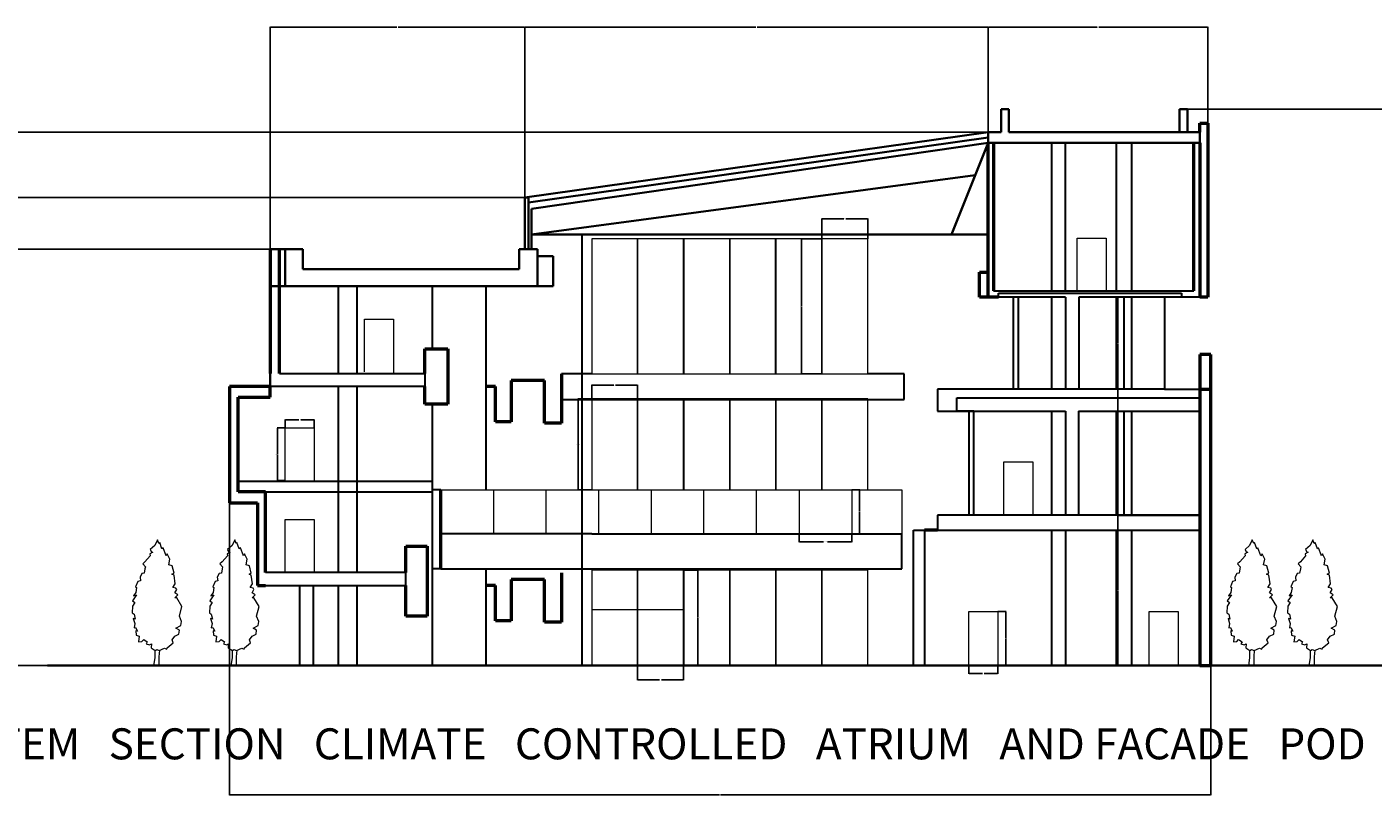
# Model space of a CAD drawing. Units: inches. Extents: x -934 to 898, y -1502 to 444.
# Tile 6 of 10: x -511 to 286, y -735 to -280. Entities that reach past the tile are written whole.
import ezdxf

# ---------------------------------------------------------------- set-up
doc = ezdxf.new("R2010")
doc.units = ezdxf.units.IN
doc.header["$MEASUREMENT"] = 0
for name, color, linetype, lineweight in [('A-ANNO-DIMS', 2, 'Continuous', 18), ('A-ANNO-TITL', 7, 'Continuous', 30), ('A-COLS', 1, 'Continuous', 30), ('A-DOOR', 3, 'Continuous', 18), ('A-FLOR', 7, 'Continuous', 30), ('A-GLAZ', 4, 'Continuous', 13), ('A-ROOF', 7, 'Continuous', 35), ('A-SECT', 7, 'Continuous', 50), ('L-GRND', 7, 'Continuous', 35), ('L-PLNT-TREE', 3, 'Continuous', 13)]:
    doc.layers.add(name, color=color, linetype=linetype, lineweight=lineweight)
doc.styles.get("Standard").update_dxf_attribs({"font": 'arial.ttf'})
doc.dimstyles.get("Standard").update_dxf_attribs({"dimtxt": 0.18, "dimasz": 0.18, "dimexe": 0.18, "dimexo": 0.0625, "dimgap": 0.09, "dimtad": 0, "dimtih": 1, "dimtoh": 1, "dimdec": 4, "dimzin": 0, "dimdsep": 46, "dimtxsty": 'Standard', "dimcen": 0.09, "dimadec": 0, "dimazin": 0, "dimtfac": 1, "dimtdec": 4, "dimtofl": 0, "dimtmove": 0, "dimatfit": 3, "dimfxl": 1, "dimtolj": 1, "dimtzin": 0, "dimarcsym": 0})

# ---------------------------------------------------------------- blocks, each defined once
blk = doc.blocks.new('*U5')
blk.add_lwpolyline([(-2.754, 191.699), (-6.78, 182.851), (-13.682, 176.953), (-11.956, 173.266), (-9.656, 172.529), (-14.257, 170.317), (-13.682, 167.368), (-21.733, 157.783), (-25.184, 154.834), (-21.158, 150.41), (-21.733, 147.461), (-22.884, 140.825), (-26.334, 140.087), (-29.21, 134.926), (-28.635, 129.028), (-32.661, 128.291), (-36.111, 120.18), (-34.386, 118.706), (-35.536, 111.333), (-38.987, 106.171), (-34.386, 107.646), (-40.712, 98.798), (-37.261, 95.849), (-40.712, 90.688), (-41.287, 80.366), (-38.412, 78.154), (-36.686, 70.781), (-39.562, 71.518), (-37.261, 64.145), (-38.412, 57.509), (-36.111, 58.247), (-33.236, 52.348), (-35.536, 53.086), (-34.961, 46.45), (-30.36, 44.975), (-31.51, 36.128), (-26.334, 36.865), (-23.459, 39.814), (-18.283, 36.128), (-20.008, 33.178), (-14.832, 31.704), (-11.956, 33.178), (-12.531, 27.28), (-6.205, 22.856), (-3.905, 24.331), (0.121, 22.856), (8.173, 26.543), (11.624, 25.068), (12.199, 27.28), (21.4, 34.653), (19.675, 39.077), (23.701, 44.975), (30.027, 47.924), (30.602, 53.823), (25.426, 56.772), (32.903, 61.196), (34.053, 67.094), (30.602, 75.205), (34.628, 89.951), (26.576, 103.222), (23.701, 103.222), (28.302, 107.646), (23.701, 110.595), (26.576, 115.756), (25.426, 117.968), (20.825, 118.706), (24.276, 124.604), (22.551, 137.876), (19.1, 139.35), (22.551, 140.825), (19.675, 151.884), (14.499, 153.359), (16.224, 162.207), (12.199, 170.317), (10.473, 167.368), (5.872, 179.165), (4.147, 177.69), (0.696, 187.275), (-0.454, 185.8)], close=True)
for points in [[(-6.813, 23.669), (-6.813, 11.669), (-8.627, 0)], [(0.387, 23.669), (-0.576, 13.271), (-0.576, 3.686), (0, 0)]]:
    blk.add_lwpolyline(points)
blk = doc.blocks.new('ATRIUM-GLAZ-UPPER')
for p, q in [((27.19, 79.9), (0, 79.9)), ((0, 79.9), (0, 0)), ((27.19, 0), (27.19, 79.9)), ((0, 0), (27.19, 0))]:
    blk.add_line(p, q)
blk = doc.blocks.new('ATRIUM-GLAZ-MIDDLE')
for p, q in [((0, 53.77), (0, 0)), ((27.19, 53.77), (0, 53.77)), ((27.19, 0), (27.19, 53.77))]:
    blk.add_line(p, q)
blk = doc.blocks.new('ATRIUM-GLAZ-LOWER')
for p, q in [((0, 56.46), (0, 0)), ((27.19, 56.46), (0, 56.46)), ((27.19, 0), (27.19, 56.46))]:
    blk.add_line(p, q)
blk = doc.blocks.new('ATRIUM-PARAPET-PANEL')
for p, q in [((0, 26.13), (31.1, 26.13)), ((31.1, 26.13), (31.1, 0))]:
    blk.add_line(p, q)
blk = doc.blocks.new('DOOR-SECT-WING')
for p, q in [((0, 0.03), (0, 31.28)), ((0, 31.28), (17.18, 31.28)), ((17.18, 31.28), (17.18, 0))]:
    blk.add_line(p, q)
blk = doc.blocks.new('DOOR-SECT-GROUND')
for p, q in [((0, 0.71), (0, 31.96)), ((0, 31.96), (17.18, 31.96)), ((17.18, 31.96), (17.18, 0))]:
    blk.add_line(p, q)
blk = doc.blocks.new('*D47')
at = {"layer": 'A-ANNO-DIMS', "color": 0, "lineweight": -2, "transparency": 16777216}
for p, q in [((-53.61, -580.06), (-53.61, -584.84)), ((-22.51, -580.06), (-22.51, -584.84)), ((-53.43, -584.66), (-39.21, -584.66)), ((-22.69, -584.66), (-36.92, -584.66))]:
    blk.add_line(p, q, dxfattribs=at)
at = {"layer": 'A-ANNO-DIMS', "color": 0, "transparency": 16777216}
for points in [[(-53.43, -584.63), (-53.43, -584.69), (-53.61, -584.66)], [(-22.69, -584.63), (-22.69, -584.69), (-22.51, -584.66)]]:
    blk.add_solid(points, dxfattribs=at)
at = {"layer": 'Defpoints', "color": 0, "transparency": 16777216}
for p in [(-53.61, -579.99), (-22.51, -579.99), (-22.51, -584.66)]:
    blk.add_point(p, dxfattribs=at)
at = {"layer": 'A-ANNO-DIMS', "color": 0, "transparency": 16777216, "insert": (-38.06, -584.66), "char_height": 0.18, "attachment_point": 5}
blk.add_mtext('\\A1;PARAPET 31 TYP.', dxfattribs=at)
blk = doc.blocks.new('*D48')
at = {"layer": 'A-ANNO-DIMS', "color": 0, "lineweight": -2, "transparency": 16777216}
for p, q in [((-22.45, -553.87), (-17.67, -553.87)), ((-17.85, -554.05), (-17.85, -566.75)), ((-17.85, -579.81), (-17.85, -567.11)), ((-22.45, -579.99), (-17.67, -579.99))]:
    blk.add_line(p, q, dxfattribs=at)
at = {"layer": 'A-ANNO-DIMS', "color": 0, "transparency": 16777216}
for points in [[(-17.88, -554.05), (-17.82, -554.05), (-17.85, -553.87)], [(-17.88, -579.81), (-17.82, -579.81), (-17.85, -579.99)]]:
    blk.add_solid(points, dxfattribs=at)
at = {"layer": 'Defpoints', "color": 0, "transparency": 16777216}
for p in [(-22.51, -553.87), (-17.85, -553.87), (-22.51, -579.99)]:
    blk.add_point(p, dxfattribs=at)
at = {"layer": 'A-ANNO-DIMS', "color": 0, "transparency": 16777216, "insert": (-17.85, -566.93), "char_height": 0.18, "attachment_point": 5}
blk.add_mtext('\\A1;26 TYP.', dxfattribs=at)
blk = doc.blocks.new('*D49')
at = {"layer": 'A-ANNO-DIMS', "color": 0, "lineweight": -2, "transparency": 16777216}
for p, q in [((-40.27, -405.38), (-52.38, -405.38)), ((-52.2, -405.56), (-52.2, -445.15)), ((-52.2, -485.1), (-52.2, -445.51)), ((-40.27, -485.28), (-52.38, -485.28))]:
    blk.add_line(p, q, dxfattribs=at)
at = {"layer": 'A-ANNO-DIMS', "color": 0, "transparency": 16777216}
for points in [[(-52.23, -405.56), (-52.17, -405.56), (-52.2, -405.38)], [(-52.23, -485.1), (-52.17, -485.1), (-52.2, -485.28)]]:
    blk.add_solid(points, dxfattribs=at)
at = {"layer": 'Defpoints', "color": 0, "transparency": 16777216}
for p in [(-40.21, -405.38), (-52.2, -485.28), (-40.21, -485.28)]:
    blk.add_point(p, dxfattribs=at)
at = {"layer": 'A-ANNO-DIMS', "color": 0, "transparency": 16777216, "insert": (-52.2, -445.33), "char_height": 0.18, "attachment_point": 5}
blk.add_mtext('\\A1;UPPER LIGHT 80 TYP.', dxfattribs=at)
blk = doc.blocks.new('*D50')
at = {"layer": 'A-ANNO-DIMS', "color": 0, "lineweight": -2, "transparency": 16777216}
for p, q in [((-40.21, -405.32), (-40.21, -393.22)), ((-40.03, -393.4), (-27.15, -393.4)), ((-13.21, -393.4), (-26.09, -393.4)), ((-13.03, -405.32), (-13.03, -393.22))]:
    blk.add_line(p, q, dxfattribs=at)
at = {"layer": 'A-ANNO-DIMS', "color": 0, "transparency": 16777216}
for points in [[(-40.03, -393.37), (-40.03, -393.43), (-40.21, -393.4)], [(-13.21, -393.37), (-13.21, -393.43), (-13.03, -393.4)]]:
    blk.add_solid(points, dxfattribs=at)
at = {"layer": 'Defpoints', "color": 0, "transparency": 16777216}
for p in [(-40.21, -393.4), (-40.21, -405.38), (-13.03, -405.38)]:
    blk.add_point(p, dxfattribs=at)
at = {"layer": 'A-ANNO-DIMS', "color": 0, "transparency": 16777216, "insert": (-26.62, -393.4), "char_height": 0.18, "attachment_point": 5}
blk.add_mtext('\\A1;27 TYP.', dxfattribs=at)
blk = doc.blocks.new('*D51')
at = {"layer": 'A-ANNO-DIMS', "color": 0, "lineweight": -2, "transparency": 16777216}
for p, q in [((-176.56, -500.1), (-184.74, -500.1)), ((-184.56, -500.28), (-184.56, -526.8)), ((-184.56, -553.69), (-184.56, -527.17)), ((-176.56, -553.87), (-184.74, -553.87))]:
    blk.add_line(p, q, dxfattribs=at)
at = {"layer": 'A-ANNO-DIMS', "color": 0, "transparency": 16777216}
for points in [[(-184.59, -500.28), (-184.53, -500.28), (-184.56, -500.1)], [(-184.59, -553.69), (-184.53, -553.69), (-184.56, -553.87)]]:
    blk.add_solid(points, dxfattribs=at)
at = {"layer": 'Defpoints', "color": 0, "transparency": 16777216}
for p in [(-184.56, -500.1), (-176.5, -500.1), (-176.5, -553.87)]:
    blk.add_point(p, dxfattribs=at)
at = {"layer": 'A-ANNO-DIMS', "color": 0, "transparency": 16777216, "insert": (-184.56, -526.98), "char_height": 0.18, "attachment_point": 5}
blk.add_mtext('\\A1;MIDDLE LIGHT 54 TYP.', dxfattribs=at)
blk = doc.blocks.new('*D52')
at = {"layer": 'A-ANNO-DIMS', "color": 0, "lineweight": -2, "transparency": 16777216}
for p, q in [((-176.5, -500.04), (-176.5, -491.85)), ((-176.32, -492.03), (-163.44, -492.03)), ((-149.49, -492.03), (-162.38, -492.03)), ((-149.31, -500.04), (-149.31, -491.85))]:
    blk.add_line(p, q, dxfattribs=at)
at = {"layer": 'A-ANNO-DIMS', "color": 0, "transparency": 16777216}
for points in [[(-176.32, -492), (-176.32, -492.06), (-176.5, -492.03)], [(-149.49, -492), (-149.49, -492.06), (-149.31, -492.03)]]:
    blk.add_solid(points, dxfattribs=at)
at = {"layer": 'Defpoints', "color": 0, "transparency": 16777216}
for p in [(-149.31, -492.03), (-176.5, -500.1), (-149.31, -500.1)]:
    blk.add_point(p, dxfattribs=at)
at = {"layer": 'A-ANNO-DIMS', "color": 0, "transparency": 16777216, "insert": (-162.91, -492.03), "char_height": 0.18, "attachment_point": 5}
blk.add_mtext('\\A1;27 TYP.', dxfattribs=at)
blk = doc.blocks.new('*D53')
at = {"layer": 'A-ANNO-DIMS', "color": 0, "lineweight": -2, "transparency": 16777216}
for p, q in [((-122.06, -601.55), (-113.48, -601.55)), ((-113.66, -601.73), (-113.66, -629.59)), ((-113.66, -657.82), (-113.66, -629.96)), ((-122.06, -658), (-113.48, -658))]:
    blk.add_line(p, q, dxfattribs=at)
at = {"layer": 'A-ANNO-DIMS', "color": 0, "transparency": 16777216}
for points in [[(-113.69, -601.73), (-113.63, -601.73), (-113.66, -601.55)], [(-113.69, -657.82), (-113.63, -657.82), (-113.66, -658)]]:
    blk.add_solid(points, dxfattribs=at)
at = {"layer": 'Defpoints', "color": 0, "transparency": 16777216}
for p in [(-122.13, -601.55), (-113.66, -601.55), (-122.13, -658)]:
    blk.add_point(p, dxfattribs=at)
at = {"layer": 'A-ANNO-DIMS', "color": 0, "transparency": 16777216, "insert": (-113.66, -629.77), "char_height": 0.18, "attachment_point": 5}
blk.add_mtext('\\A1;LOWER LIGHT 56 TYP.', dxfattribs=at)
blk = doc.blocks.new('*D54')
at = {"layer": 'A-ANNO-DIMS', "color": 0, "lineweight": -2, "transparency": 16777216}
for p, q in [((-149.31, -658.07), (-149.31, -666.65)), ((-122.13, -658.07), (-122.13, -666.65)), ((-149.13, -666.47), (-136.25, -666.47)), ((-122.31, -666.47), (-135.19, -666.47))]:
    blk.add_line(p, q, dxfattribs=at)
at = {"layer": 'A-ANNO-DIMS', "color": 0, "transparency": 16777216}
for points in [[(-149.13, -666.44), (-149.13, -666.5), (-149.31, -666.47)], [(-122.31, -666.44), (-122.31, -666.5), (-122.13, -666.47)]]:
    blk.add_solid(points, dxfattribs=at)
at = {"layer": 'Defpoints', "color": 0, "transparency": 16777216}
for p in [(-149.31, -658), (-122.13, -658), (-122.13, -666.47)]:
    blk.add_point(p, dxfattribs=at)
at = {"layer": 'A-ANNO-DIMS', "color": 0, "transparency": 16777216, "insert": (-135.72, -666.47), "char_height": 0.18, "attachment_point": 5}
blk.add_mtext('\\A1;27 TYP.', dxfattribs=at)
blk = doc.blocks.new('*D55')
at = {"layer": 'A-ANNO-DIMS', "color": 0, "lineweight": -2, "transparency": 16777216}
for p, q in [((64.03, -626.04), (68.95, -626.04)), ((68.77, -626.22), (68.77, -641.84)), ((68.77, -657.82), (68.77, -642.2)), ((64.03, -658), (68.95, -658))]:
    blk.add_line(p, q, dxfattribs=at)
at = {"layer": 'A-ANNO-DIMS', "color": 0, "transparency": 16777216}
for points in [[(68.74, -626.22), (68.8, -626.22), (68.77, -626.04)], [(68.74, -657.82), (68.8, -657.82), (68.77, -658)]]:
    blk.add_solid(points, dxfattribs=at)
at = {"layer": 'Defpoints', "color": 0, "transparency": 16777216}
for p in [(63.97, -626.04), (68.77, -626.04), (63.97, -658)]:
    blk.add_point(p, dxfattribs=at)
at = {"layer": 'A-ANNO-DIMS', "color": 0, "transparency": 16777216, "insert": (68.77, -642.02), "char_height": 0.18, "attachment_point": 5}
blk.add_mtext('\\A1;ENTRY 32 TYP.', dxfattribs=at)
blk = doc.blocks.new('*D56')
at = {"layer": 'A-ANNO-DIMS', "color": 0, "lineweight": -2, "transparency": 16777216}
for p, q in [((46.79, -658.07), (46.79, -662.98)), ((63.97, -658.07), (63.97, -662.98)), ((46.97, -662.8), (54.86, -662.8)), ((63.79, -662.8), (55.9, -662.8))]:
    blk.add_line(p, q, dxfattribs=at)
at = {"layer": 'A-ANNO-DIMS', "color": 0, "transparency": 16777216}
for points in [[(46.97, -662.77), (46.97, -662.83), (46.79, -662.8)], [(63.79, -662.77), (63.79, -662.83), (63.97, -662.8)]]:
    blk.add_solid(points, dxfattribs=at)
at = {"layer": 'Defpoints', "color": 0, "transparency": 16777216}
for p in [(46.79, -658), (63.97, -658), (63.97, -662.8)]:
    blk.add_point(p, dxfattribs=at)
at = {"layer": 'A-ANNO-DIMS', "color": 0, "transparency": 16777216, "insert": (55.38, -662.8), "char_height": 0.18, "attachment_point": 5}
blk.add_mtext('\\A1;17 TYP.', dxfattribs=at)
blk = doc.blocks.new('*D57')
at = {"layer": 'A-ANNO-DIMS', "color": 0, "lineweight": -2, "transparency": 16777216}
for p, q in [((-357.96, -517.2), (-362.77, -517.2)), ((-362.59, -517.38), (-362.59, -532.66)), ((-362.59, -548.3), (-362.59, -533.03)), ((-357.96, -548.48), (-362.77, -548.48))]:
    blk.add_line(p, q, dxfattribs=at)
at = {"layer": 'A-ANNO-DIMS', "color": 0, "transparency": 16777216}
for points in [[(-362.62, -517.38), (-362.56, -517.38), (-362.59, -517.2)], [(-362.62, -548.3), (-362.56, -548.3), (-362.59, -548.48)]]:
    blk.add_solid(points, dxfattribs=at)
at = {"layer": 'Defpoints', "color": 0, "transparency": 16777216}
for p in [(-362.59, -517.2), (-357.9, -517.2), (-357.9, -548.48)]:
    blk.add_point(p, dxfattribs=at)
at = {"layer": 'A-ANNO-DIMS', "color": 0, "transparency": 16777216, "insert": (-362.59, -532.84), "char_height": 0.18, "attachment_point": 5}
blk.add_mtext('\\A1;WING DOOR 31 TYP.', dxfattribs=at)
blk = doc.blocks.new('*D58')
at = {"layer": 'A-ANNO-DIMS', "color": 0, "lineweight": -2, "transparency": 16777216}
for p, q in [((-357.9, -517.14), (-357.9, -512.33)), ((-357.72, -512.51), (-349.82, -512.51)), ((-340.89, -512.51), (-348.78, -512.51)), ((-340.71, -517.14), (-340.71, -512.33))]:
    blk.add_line(p, q, dxfattribs=at)
at = {"layer": 'A-ANNO-DIMS', "color": 0, "transparency": 16777216}
for points in [[(-357.72, -512.48), (-357.72, -512.54), (-357.9, -512.51)], [(-340.89, -512.48), (-340.89, -512.54), (-340.71, -512.51)]]:
    blk.add_solid(points, dxfattribs=at)
at = {"layer": 'Defpoints', "color": 0, "transparency": 16777216}
for p in [(-357.9, -517.2), (-340.71, -512.51), (-340.71, -517.2)]:
    blk.add_point(p, dxfattribs=at)
at = {"layer": 'A-ANNO-DIMS', "color": 0, "transparency": 16777216, "insert": (-349.3, -512.51), "char_height": 0.18, "attachment_point": 5}
blk.add_mtext('\\A1;17 TYP.', dxfattribs=at)
blk = doc.blocks.new('*D97')
at = {"layer": 'A-ANNO-DIMS', "color": 0, "lineweight": -2, "transparency": 16777216}
for p, q in [((-391.01, -492.82), (-391.01, -734.71)), ((190.03, -658.07), (190.03, -734.71)), ((-390.83, -734.53), (-100.76, -734.53)), ((189.85, -734.53), (-100.22, -734.53))]:
    blk.add_line(p, q, dxfattribs=at)
at = {"layer": 'A-ANNO-DIMS', "color": 0, "transparency": 16777216}
for points in [[(-390.83, -734.5), (-390.83, -734.56), (-391.01, -734.53)], [(189.85, -734.5), (189.85, -734.56), (190.03, -734.53)]]:
    blk.add_solid(points, dxfattribs=at)
at = {"layer": 'Defpoints', "color": 0, "transparency": 16777216}
for p in [(-391.01, -492.76), (190.03, -658), (190.03, -734.53)]:
    blk.add_point(p, dxfattribs=at)
at = {"layer": 'A-ANNO-DIMS', "color": 0, "transparency": 16777216, "insert": (-100.49, -734.53), "char_height": 0.18, "attachment_point": 5}
blk.add_mtext('\\A1;581', dxfattribs=at)
blk = doc.blocks.new('*D98')
at = {"layer": 'A-ANNO-DIMS', "color": 0, "lineweight": -2, "transparency": 16777216}
for p, q in [((176.35, -328.53), (343, -328.53)), ((342.82, -328.71), (342.82, -493.08)), ((342.82, -657.82), (342.82, -493.45)), ((190.1, -658), (343, -658))]:
    blk.add_line(p, q, dxfattribs=at)
at = {"layer": 'A-ANNO-DIMS', "color": 0, "transparency": 16777216}
for points in [[(342.79, -328.71), (342.85, -328.71), (342.82, -328.53)], [(342.79, -657.82), (342.85, -657.82), (342.82, -658)]]:
    blk.add_solid(points, dxfattribs=at)
at = {"layer": 'Defpoints', "color": 0, "transparency": 16777216}
for p in [(176.29, -328.53), (342.82, -328.53), (190.03, -658)]:
    blk.add_point(p, dxfattribs=at)
at = {"layer": 'A-ANNO-DIMS', "color": 0, "transparency": 16777216, "insert": (342.82, -493.26), "char_height": 0.18, "attachment_point": 5}
blk.add_mtext('\\A1;329.5', dxfattribs=at)
blk = doc.blocks.new('*D99')
at = {"layer": 'A-ANNO-DIMS', "color": 0, "lineweight": -2, "transparency": 16777216}
for p, q in [((-216.13, -380.72), (-216.13, -279.8)), ((-215.95, -279.98), (-79.37, -279.98)), ((58, -279.98), (-78.58, -279.98)), ((58.18, -342.04), (58.18, -279.8))]:
    blk.add_line(p, q, dxfattribs=at)
at = {"layer": 'A-ANNO-DIMS', "color": 0, "transparency": 16777216}
for points in [[(-215.95, -279.95), (-215.95, -280.01), (-216.13, -279.98)], [(58, -279.95), (58, -280.01), (58.18, -279.98)]]:
    blk.add_solid(points, dxfattribs=at)
at = {"layer": 'Defpoints', "color": 0, "transparency": 16777216}
for p in [(58.18, -279.98), (58.18, -342.1), (-216.13, -380.79)]:
    blk.add_point(p, dxfattribs=at)
at = {"layer": 'A-ANNO-DIMS', "color": 0, "transparency": 16777216, "insert": (-78.97, -279.98), "char_height": 0.18, "attachment_point": 5}
blk.add_mtext('\\A1;274.3', dxfattribs=at)
blk = doc.blocks.new('*D100')
at = {"layer": 'A-ANNO-DIMS', "color": 0, "lineweight": -2, "transparency": 16777216}
for p, q in [((58.18, -342.04), (58.18, -279.8)), ((58.36, -279.98), (122.81, -279.98)), ((188.17, -279.98), (123.72, -279.98)), ((188.35, -336.73), (188.35, -279.8))]:
    blk.add_line(p, q, dxfattribs=at)
at = {"layer": 'A-ANNO-DIMS', "color": 0, "transparency": 16777216}
for points in [[(58.36, -279.95), (58.36, -280.01), (58.18, -279.98)], [(188.17, -279.95), (188.17, -280.01), (188.35, -279.98)]]:
    blk.add_solid(points, dxfattribs=at)
at = {"layer": 'Defpoints', "color": 0, "transparency": 16777216}
for p in [(188.35, -279.98), (58.18, -342.1), (188.35, -336.79)]:
    blk.add_point(p, dxfattribs=at)
at = {"layer": 'A-ANNO-DIMS', "color": 0, "transparency": 16777216, "insert": (123.26, -279.98), "char_height": 0.18, "attachment_point": 5}
blk.add_mtext('\\A1;130.17', dxfattribs=at)
blk = doc.blocks.new('*D101')
at = {"layer": 'A-ANNO-DIMS', "color": 0, "lineweight": -2, "transparency": 16777216}
for p, q in [((183.53, -569.04), (134.86, -569.04)), ((135.04, -569.22), (135.04, -613.34)), ((135.04, -657.82), (135.04, -613.7)), ((183.53, -658), (134.86, -658))]:
    blk.add_line(p, q, dxfattribs=at)
at = {"layer": 'A-ANNO-DIMS', "color": 0, "transparency": 16777216}
for points in [[(135.01, -569.22), (135.07, -569.22), (135.04, -569.04)], [(135.01, -657.82), (135.07, -657.82), (135.04, -658)]]:
    blk.add_solid(points, dxfattribs=at)
at = {"layer": 'Defpoints', "color": 0, "transparency": 16777216}
for p in [(135.04, -569.04), (183.59, -569.04), (183.59, -658)]:
    blk.add_point(p, dxfattribs=at)
at = {"layer": 'A-ANNO-DIMS', "color": 0, "transparency": 16777216, "insert": (135.04, -613.52), "char_height": 0.18, "attachment_point": 5}
blk.add_mtext('\\A1;88.97', dxfattribs=at)
blk = doc.blocks.new('*D102')
at = {"layer": 'A-ANNO-DIMS', "color": 0, "lineweight": -2, "transparency": 16777216}
for p, q in [((183.53, -494.41), (134.86, -494.41)), ((135.04, -494.59), (135.04, -531.54)), ((135.04, -568.86), (135.04, -531.91)), ((183.53, -569.04), (134.86, -569.04))]:
    blk.add_line(p, q, dxfattribs=at)
at = {"layer": 'A-ANNO-DIMS', "color": 0, "transparency": 16777216}
for points in [[(135.01, -494.59), (135.07, -494.59), (135.04, -494.41)], [(135.01, -568.86), (135.07, -568.86), (135.04, -569.04)]]:
    blk.add_solid(points, dxfattribs=at)
at = {"layer": 'Defpoints', "color": 0, "transparency": 16777216}
for p in [(135.04, -494.41), (183.59, -494.41), (183.59, -569.04)]:
    blk.add_point(p, dxfattribs=at)
at = {"layer": 'A-ANNO-DIMS', "color": 0, "transparency": 16777216, "insert": (135.04, -531.72), "char_height": 0.18, "attachment_point": 5}
blk.add_mtext('\\A1;74.63', dxfattribs=at)
blk = doc.blocks.new('*D103')
at = {"layer": 'A-ANNO-DIMS', "color": 0, "lineweight": -2, "transparency": 16777216}
for p, q in [((183.53, -439.81), (134.86, -439.81)), ((135.04, -439.99), (135.04, -466.93)), ((135.04, -494.23), (135.04, -467.29)), ((183.53, -494.41), (134.86, -494.41))]:
    blk.add_line(p, q, dxfattribs=at)
at = {"layer": 'A-ANNO-DIMS', "color": 0, "transparency": 16777216}
for points in [[(135.01, -439.99), (135.07, -439.99), (135.04, -439.81)], [(135.01, -494.23), (135.07, -494.23), (135.04, -494.41)]]:
    blk.add_solid(points, dxfattribs=at)
at = {"layer": 'Defpoints', "color": 0, "transparency": 16777216}
for p in [(135.04, -439.81), (183.59, -439.81), (183.59, -494.41)]:
    blk.add_point(p, dxfattribs=at)
at = {"layer": 'A-ANNO-DIMS', "color": 0, "transparency": 16777216, "insert": (135.04, -467.11), "char_height": 0.18, "attachment_point": 5}
blk.add_mtext('\\A1;54.61', dxfattribs=at)
blk = doc.blocks.new('*D104')
at = {"layer": 'A-ANNO-DIMS', "color": 0, "lineweight": -2, "transparency": 16777216}
for p, q in [((-366.82, -411.42), (-366.82, -279.8)), ((-366.64, -279.98), (-291.86, -279.98)), ((-216.31, -279.98), (-291.09, -279.98)), ((-216.13, -380.72), (-216.13, -279.8))]:
    blk.add_line(p, q, dxfattribs=at)
at = {"layer": 'A-ANNO-DIMS', "color": 0, "transparency": 16777216}
for points in [[(-366.64, -279.95), (-366.64, -280.01), (-366.82, -279.98)], [(-216.31, -279.95), (-216.31, -280.01), (-216.13, -279.98)]]:
    blk.add_solid(points, dxfattribs=at)
at = {"layer": 'Defpoints', "color": 0, "transparency": 16777216}
for p in [(-216.13, -279.98), (-216.13, -380.79), (-366.82, -411.48)]:
    blk.add_point(p, dxfattribs=at)
at = {"layer": 'A-ANNO-DIMS', "color": 0, "transparency": 16777216, "insert": (-291.47, -279.98), "char_height": 0.18, "attachment_point": 5}
blk.add_mtext('\\A1;150.7', dxfattribs=at)
blk = doc.blocks.new('*D105')
at = {"layer": 'A-ANNO-DIMS', "color": 0, "lineweight": -2, "transparency": 16777216}
for p, q in [((-366.88, -411.48), (-547.37, -411.48)), ((-547.19, -411.66), (-547.19, -534.56)), ((-547.19, -657.82), (-547.19, -534.93)), ((-349.49, -658), (-547.37, -658))]:
    blk.add_line(p, q, dxfattribs=at)
at = {"layer": 'A-ANNO-DIMS', "color": 0, "transparency": 16777216}
for points in [[(-547.22, -411.66), (-547.16, -411.66), (-547.19, -411.48)], [(-547.22, -657.82), (-547.16, -657.82), (-547.19, -658)]]:
    blk.add_solid(points, dxfattribs=at)
at = {"layer": 'Defpoints', "color": 0, "transparency": 16777216}
for p in [(-547.19, -411.48), (-366.82, -411.48), (-349.43, -658)]:
    blk.add_point(p, dxfattribs=at)
at = {"layer": 'A-ANNO-DIMS', "color": 0, "transparency": 16777216, "insert": (-547.19, -534.74), "char_height": 0.18, "attachment_point": 5}
blk.add_mtext('\\A1;246.5', dxfattribs=at)
blk = doc.blocks.new('*D106')
at = {"layer": 'A-ANNO-DIMS', "color": 0, "lineweight": -2, "transparency": 16777216}
for p, q in [((58.12, -342.1), (-547.37, -342.1)), ((-547.19, -342.28), (-547.19, -361.26)), ((-547.19, -380.61), (-547.19, -361.63)), ((-216.19, -380.79), (-547.37, -380.79))]:
    blk.add_line(p, q, dxfattribs=at)
at = {"layer": 'A-ANNO-DIMS', "color": 0, "transparency": 16777216}
for points in [[(-547.22, -342.28), (-547.16, -342.28), (-547.19, -342.1)], [(-547.22, -380.61), (-547.16, -380.61), (-547.19, -380.79)]]:
    blk.add_solid(points, dxfattribs=at)
at = {"layer": 'Defpoints', "color": 0, "transparency": 16777216}
for p in [(-547.19, -342.1), (58.18, -342.1), (-216.13, -380.79)]:
    blk.add_point(p, dxfattribs=at)
at = {"layer": 'A-ANNO-DIMS', "color": 0, "transparency": 16777216, "insert": (-547.19, -361.44), "char_height": 0.18, "attachment_point": 5}
blk.add_mtext('\\A1;38.685', dxfattribs=at)

msp = doc.modelspace()

# ---------------------------------------------------------------- linework, layer by layer
at = {"layer": 'A-COLS'}
for p, q in [((95.7615, -348.4081), (95.7615, -436.1061)), ((103.9777, -436.1061), (103.9777, -348.4081)), ((133.9329, -348.4081), (133.9329, -436.1061)), ((143.0188, -348.4081), (143.0188, -436.1061)), ((-182.3834, -402.7575), (-182.3834, -658.003)), ((-326.6271, -433.3984), (-326.6271, -484.9496)), ((-315.5585, -433.3984), (-315.5585, -484.9496)), ((-270.9968, -433.3984), (-270.9968, -470.4844)), ((-239.0879, -433.3984), (-239.0879, -553.8664)), ((73.3031, -494.4116), (73.3031, -439.806)), ((75.961, -439.806), (75.961, -494.4116)), ((95.7615, -439.806), (95.7615, -494.4116)), ((103.9777, -439.806), (103.9777, -494.4116)), ((111.8674, -439.806), (111.8674, -494.4116)), ((133.9329, -439.806), (133.9329, -494.4116)), ((138.5307, -439.806), (138.5307, -494.4116)), ((143.0188, -439.806), (143.0188, -494.4116)), ((162.68, -439.806), (162.68, -494.4116)), ((-326.6271, -492.7573), (-326.6271, -602.8367)), ((-315.5585, -492.7573), (-315.5585, -602.8367)), ((-270.9968, -503.2023), (-270.9968, -658.003)), ((46.7576, -507.2543), (46.7576, -569.0379)), ((49.6617, -569.0379), (49.6617, -507.2543)), ((95.7615, -507.2543), (95.7615, -569.0379)), ((103.9777, -507.2543), (103.9777, -569.0379)), ((103.9777, -507.2543), (103.9777, -569.0379)), ((111.8018, -507.2543), (111.8018, -569.0379)), ((133.9329, -507.2543), (133.9329, -569.0379)), ((138.5307, -507.2543), (138.5307, -569.0379)), ((143.0188, -507.2543), (143.0188, -569.0379)), ((13.9725, -658.003), (13.9725, -577.8106)), ((13.9725, -577.8106), (20.5119, -577.8106)), ((20.5119, -577.8106), (20.5119, -658.003)), ((95.7615, -577.8106), (95.7615, -658.003)), ((103.9777, -577.8106), (103.9777, -658.003)), ((133.9329, -577.8106), (133.9329, -658.003)), ((143.0188, -577.8106), (143.0188, -658.003)), ((-239.0879, -600.6964), (-239.0879, -658.003)), ((-349.4313, -610.6523), (-349.4313, -658.003)), ((-341.3362, -610.6523), (-341.3362, -658.003)), ((-326.6271, -610.6523), (-326.6271, -658.003)), ((-315.5585, -610.6523), (-315.5585, -658.003))]:
    msp.add_line(p, q, dxfattribs=at)
at = {"layer": 'A-DOOR'}
for p, q in [((110.9454, -436.0725), (110.9454, -404.8225)), ((110.9454, -404.8225), (128.1279, -404.8225)), ((128.1279, -404.8225), (128.1279, -436.1061)), ((-311.02, -484.0351), (-311.02, -452.7851)), ((-311.02, -452.7851), (-293.8375, -452.7851)), ((-293.8375, -452.7851), (-293.8375, -484.9496)), ((67.5722, -568.5387), (67.5722, -537.2887)), ((67.5722, -537.2887), (84.7547, -537.2887)), ((84.7547, -537.2887), (84.7547, -569.0379))]:
    msp.add_line(p, q, dxfattribs=at)
at = {"layer": 'A-FLOR'}
for p, q in [((61.3886, -436.1061), (179.8982, -436.1061)), ((64.2799, -439.806), (64.2799, -437.5618)), ((64.2799, -437.5618), (172.6123, -437.5618)), ((172.6123, -437.5618), (172.6123, -439.806)), ((103.9777, -439.806), (58.1805, -439.806)), ((183.5947, -439.806), (111.8674, -439.806)), ((-366.8176, -492.7573), (-366.8176, -484.9496)), ((-366.8176, -484.9496), (-366.8176, -492.7573)), ((-361.2533, -484.9496), (-275.3431, -484.9496)), ((-275.3431, -484.9496), (-275.3431, -484.9496)), ((-275.3431, -484.9496), (-275.3431, -492.7573)), ((-176.4995, -485.2796), (-194.3343, -485.2796)), ((-194.3343, -485.2796), (-194.3343, -500.3596)), ((8.5295, -485.2796), (-13.0254, -485.2796)), ((8.5295, -500.3596), (8.5295, -485.2796)), ((-275.3431, -492.7573), (-366.8176, -492.7573)), ((-194.3343, -500.3596), (8.5295, -500.3596)), ((75.961, -494.4116), (28.2418, -494.4116)), ((28.2418, -494.4116), (28.2418, -507.2543)), ((39.6173, -507.2543), (39.6173, -499.494)), ((39.6173, -499.494), (183.5947, -499.494)), ((162.68, -494.4116), (75.961, -494.4116)), ((162.68, -494.4116), (183.5947, -494.4116)), ((183.5947, -507.2543), (183.5947, -494.4116)), ((28.2418, -507.2543), (103.9777, -507.2543)), ((49.6617, -507.2543), (39.6173, -507.2543)), ((49.6617, -507.2543), (46.7576, -507.2543)), ((49.6617, -507.2543), (49.6617, -507.2543)), ((111.8018, -507.2543), (183.5947, -507.2543)), ((-326.6271, -548.9964), (-385.7189, -548.9964)), ((-315.5585, -548.9964), (-326.6271, -548.9964)), ((-270.9968, -548.9964), (-315.5585, -548.9964)), ((-369.5114, -555.184), (-270.9968, -555.184)), ((-265.7617, -553.8664), (-270.9968, -553.8664)), ((183.5947, -569.0379), (28.2418, -569.0379)), ((28.2418, -569.0379), (28.2418, -577.8106)), ((183.5947, -577.8106), (183.5947, -569.0379)), ((-176.4995, -579.9948), (-265.7617, -579.9948)), ((-265.7617, -579.9948), (-265.7617, -600.6964)), ((-176.4995, -579.9948), (7.1993, -579.9948)), ((7.1993, -600.6964), (7.1993, -579.9948)), ((28.2418, -577.8106), (183.5947, -577.8106)), ((-286.5304, -602.8367), (-369.5114, -602.8367)), ((-286.5304, -610.6523), (-286.5304, -602.8367)), ((-265.7617, -600.6964), (-270.9968, -600.6964)), ((-265.7617, -600.6964), (7.1993, -600.6964)), ((-374.3118, -610.6523), (-286.5304, -610.6523)), ((-286.5304, -610.6523), (-286.5304, -610.6523))]:
    msp.add_line(p, q, dxfattribs=at)
at = {"layer": 'A-GLAZ'}
for p, q in [((-22.5108, -553.8664), (7.1993, -553.8664)), ((7.1993, -553.8664), (7.1993, -579.9948)), ((-176.4995, -624.7684), (-121.9486, -624.7684))]:
    msp.add_line(p, q, dxfattribs=at)
at = {"layer": 'A-ROOF'}
for p, q in [((65.953, -328.5269), (65.953, -342.1362)), ((65.953, -328.5269), (70.5216, -328.5269)), ((70.5216, -328.5269), (70.5216, -342.1018)), ((176.286, -328.5269), (171.5496, -328.5269)), ((171.5496, -328.5269), (171.5496, -342.1362)), ((176.286, -342.1362), (176.286, -328.5269)), ((58.1805, -342.1018), (-216.1305, -380.7865)), ((58.1805, -342.1018), (58.1805, -348.4081)), ((65.953, -342.1018), (58.1805, -342.1018)), ((74.9219, -342.1018), (70.5216, -342.1018)), ((70.5216, -342.1018), (152.2251, -342.1018)), ((152.2251, -342.1018), (171.5496, -342.1018)), ((179.026, -342.1362), (161.3617, -342.1362)), ((176.286, -342.1018), (183.5947, -342.1018)), ((183.5947, -348.4081), (183.5947, -342.1018)), ((58.1805, -345.2515), (-213.9083, -383.8591)), ((58.1805, -348.4081), (-212.2172, -387.5172)), ((58.1805, -348.4081), (36.4296, -402.7575)), ((58.1805, -348.4081), (64.7167, -348.4081)), ((58.1805, -348.4081), (183.5947, -348.4081)), ((176.2414, -348.4081), (183.5947, -348.4081)), ((50.4784, -367.6536), (-212.2172, -402.7575)), ((-216.1305, -411.4835), (-216.1305, -380.7865)), ((-216.1305, -380.7865), (-213.9083, -380.7865)), ((-213.9083, -380.7865), (-213.9083, -411.4835)), ((-212.2172, -411.4835), (-212.2172, -387.5172)), ((-212.2172, -402.7575), (36.4296, -402.7575)), ((36.4296, -402.7575), (58.1805, -402.7575)), ((-366.8176, -411.4835), (-357.9265, -411.4835)), ((-357.9265, -411.4835), (-357.9265, -433.3984)), ((-357.9265, -433.3984), (-357.9265, -411.4835)), ((-357.9265, -411.4835), (-347.4096, -411.4835)), ((-347.4096, -411.4835), (-347.4096, -423.3142)), ((-219.413, -423.3142), (-219.413, -411.4835)), ((-219.413, -411.4835), (-208.5956, -411.4835)), ((-208.5956, -411.4835), (-208.5956, -423.3142)), ((-208.5956, -423.3142), (-208.5956, -415.5473)), ((-208.5956, -415.5473), (-199.3227, -415.5473)), ((-199.3227, -415.5473), (-199.3227, -423.3142)), ((-347.4096, -423.3142), (-219.413, -423.3142)), ((-208.5956, -423.3142), (-208.5956, -433.3984)), ((-199.3227, -423.3142), (-199.3227, -433.3984)), ((-357.9265, -433.3984), (-366.8176, -433.3984)), ((-199.3227, -433.3984), (-366.8176, -433.3984)), ((-357.9265, -433.3984), (-357.9265, -433.3984))]:
    msp.add_line(p, q, dxfattribs=at)
at = {"layer": 'A-SECT'}
for p, q in [((183.5947, -342.1018), (183.5947, -336.7893)), ((183.5947, -336.7893), (188.3459, -336.7893)), ((188.3459, -336.7893), (188.3459, -439.806)), ((58.1805, -439.806), (58.1805, -348.4081)), ((61.3886, -348.4081), (61.3886, -436.1061)), ((179.8982, -436.1061), (179.8982, -348.4081)), ((183.5947, -348.4081), (183.5947, -439.806)), ((-366.8176, -411.4835), (-366.8176, -456.9383)), ((-361.2533, -484.9496), (-361.2533, -411.4835)), ((53.1818, -439.806), (53.1818, -425.088)), ((53.1818, -425.088), (58.1805, -425.088)), ((64.2799, -439.806), (53.1818, -439.806)), ((188.3459, -439.806), (183.5947, -439.806)), ((-366.8176, -456.9383), (-366.8176, -484.9496)), ((-275.3431, -484.9496), (-275.3431, -470.4844)), ((-275.3431, -470.4844), (-261.7143, -470.4844)), ((-261.7143, -470.4844), (-261.7143, -503.2023)), ((190.0344, -473.6961), (183.5947, -473.6961)), ((183.5947, -473.6961), (183.5947, -494.4116)), ((190.0344, -494.4116), (190.0344, -473.6961)), ((-194.3343, -485.2796), (-194.3343, -514.4915)), ((-366.8176, -492.7573), (-391.0098, -492.7573)), ((-391.0098, -492.7573), (-391.0098, -561.7333)), ((-366.8176, -499.0567), (-366.8176, -492.7573)), ((-275.3431, -503.2023), (-275.3431, -492.7573)), ((-233.3616, -492.7573), (-239.0879, -492.7573)), ((-233.3616, -513.6556), (-233.3616, -492.7573)), ((-204.499, -489.1774), (-224.2412, -489.1774)), ((-224.2412, -489.1774), (-224.2412, -513.6556)), ((-204.499, -514.4915), (-204.499, -489.1774)), ((-385.7189, -555.184), (-385.7189, -499.0567)), ((-385.7189, -499.0567), (-366.8176, -499.0567)), ((183.5947, -494.4116), (190.0344, -494.4116)), ((183.5947, -494.4116), (183.5947, -658.003)), ((190.0344, -658.003), (190.0344, -494.4116)), ((-261.7143, -503.2023), (-275.3431, -503.2023)), ((183.5947, -507.2543), (183.5947, -569.0379)), ((-224.2412, -513.6556), (-233.3616, -513.6556)), ((-194.3343, -514.4915), (-204.499, -514.4915)), ((-369.5114, -555.184), (-385.7189, -555.184)), ((-369.5114, -561.4804), (-369.5114, -555.184)), ((-265.7617, -600.6964), (-265.7617, -553.8664)), ((-391.0098, -561.7333), (-391.0098, -561.7333)), ((-391.0098, -561.7333), (-385.7189, -561.7333)), ((-385.7189, -561.7333), (-374.3118, -561.7333)), ((-374.3118, -561.7333), (-374.3118, -610.6523)), ((-369.5114, -602.8367), (-369.5114, -561.4804)), ((28.2418, -577.8106), (20.5119, -577.8106)), ((-286.5304, -602.8367), (-286.5304, -587.2047)), ((-286.5304, -587.2047), (-273.9058, -587.2047)), ((-273.9058, -587.2047), (-273.9058, -628.6559)), ((-194.3343, -603.0798), (-194.3343, -618.1598)), ((-194.3343, -603.0798), (-194.3343, -632.2917)), ((-374.3118, -610.6523), (-369.5114, -610.6523)), ((-286.5304, -628.6559), (-286.5304, -610.6523)), ((-233.3616, -610.5575), (-239.0879, -610.5575)), ((-233.3616, -631.4558), (-233.3616, -610.5575)), ((-204.499, -606.9776), (-224.2412, -606.9776)), ((-224.2412, -606.9776), (-224.2412, -631.4558)), ((-204.499, -632.2917), (-204.499, -606.9776)), ((-273.9058, -628.6559), (-286.5304, -628.6559)), ((-224.2412, -631.4558), (-233.3616, -631.4558)), ((-194.3343, -632.2917), (-204.499, -632.2917)), ((183.5947, -658.003), (190.0344, -658.003))]:
    msp.add_line(p, q, dxfattribs=at)
at = {"layer": 'L-GRND'}
for p, q in [((183.5947, -658.003), (-498.6446, -658.003)), ((190.0344, -658.003), (294.2707, -658.003))]:
    msp.add_line(p, q, dxfattribs=at)

# ---------------------------------------------------------------- block references
at = {"layer": 'A-DOOR'}
for name, p in [('DOOR-SECT-WING', (-357.8958, -548.4832)), ('DOOR-SECT-WING', (-357.8958, -602.8367)), ('DOOR-SECT-GROUND', (46.7889, -658.003)), ('DOOR-SECT-GROUND', (153.5068, -658.003))]:
    msp.add_blockref(name, p, dxfattribs=at)
at = {"layer": 'A-GLAZ', "rotation": 180}
for p in [(-149.3133, -405.3833), (-122.1271, -405.3833), (-94.7624, -405.3833), (-67.5762, -405.3833), (-40.2116, -405.3833), (-13.0254, -405.3833)]:
    msp.add_blockref('ATRIUM-GLAZ-UPPER', p, dxfattribs=at)
at = {"layer": 'A-GLAZ'}
for name, p in [('ATRIUM-GLAZ-MIDDLE', (-176.4995, -553.8664)), ('ATRIUM-GLAZ-MIDDLE', (-149.3133, -553.8664)), ('ATRIUM-GLAZ-MIDDLE', (-121.9486, -553.8664)), ('ATRIUM-GLAZ-MIDDLE', (-94.7624, -553.8664)), ('ATRIUM-GLAZ-MIDDLE', (-67.3978, -553.8664)), ('ATRIUM-GLAZ-MIDDLE', (-40.2116, -553.8664)), ('ATRIUM-PARAPET-PANEL', (-265.7617, -579.9948)), ('ATRIUM-PARAPET-PANEL', (-234.659, -579.9948)), ('ATRIUM-PARAPET-PANEL', (-203.5563, -579.9948)), ('ATRIUM-PARAPET-PANEL', (-172.4536, -579.9948)), ('ATRIUM-PARAPET-PANEL', (-141.3509, -579.9948)), ('ATRIUM-PARAPET-PANEL', (-110.2482, -579.9948)), ('ATRIUM-PARAPET-PANEL', (-84.7162, -579.9948)), ('ATRIUM-PARAPET-PANEL', (-53.6135, -579.9948)), ('ATRIUM-GLAZ-LOWER', (-176.4995, -658.003)), ('ATRIUM-GLAZ-LOWER', (-149.3133, -658.003)), ('ATRIUM-GLAZ-LOWER', (-121.9486, -658.003)), ('ATRIUM-GLAZ-LOWER', (-94.7624, -658.003)), ('ATRIUM-GLAZ-LOWER', (-67.3978, -658.003)), ('ATRIUM-GLAZ-LOWER', (-40.2116, -658.003))]:
    msp.add_blockref(name, p, dxfattribs=at)
at = {"layer": 'L-PLNT-TREE', "xscale": 0.3888403435713332, "yscale": 0.3888403435713332, "zscale": 0.3888403435713332}
for p in [(-432.5009, -658.0261), (-386.7616, -658.0261), (215.6448, -658.0261), (251.4985, -658.0261)]:
    msp.add_blockref('*U5', p, dxfattribs=at)

# ---------------------------------------------------------------- texts
at = {"layer": 'A-ANNO-TITL'}
msp.add_text('SYSTEM   SECTION   CLIMATE   CONTROLLED   ATRIUM   AND FACADE   POD', height=18.353224, dxfattribs=at).set_placement((-572.4968, -713.5413))

# ---------------------------------------------------------------- dimensions: what is measured, and where the dimension line sits
at = {"layer": 'A-ANNO-DIMS'}
for base, p1, p2, override, picture, middle in [((-216.1305, -279.9769), (-366.8176, -411.4835), (-216.1305, -380.7865), {"dimdec": 1, "dimlfac": 1, "dimrnd": 0, "dimzin": 0, "dimdsep": 46, "dimlunit": 2}, '*D104', (-291.474, -279.9769)), ((58.1805, -279.9769), (-216.1305, -380.7865), (58.1805, -342.1018), {"dimdec": 1, "dimlfac": 1, "dimrnd": 0, "dimzin": 0, "dimdsep": 46, "dimlunit": 2}, '*D99', (-78.975, -279.9769)), ((188.3459, -279.9769), (58.1805, -342.1018), (188.3459, -336.7893), {"dimdec": 2, "dimlfac": 1, "dimrnd": 0, "dimzin": 0, "dimdsep": 46, "dimlunit": 2}, '*D100', (123.2632, -279.9769)), ((190.0344, -734.5286), (-391.0098, -492.7573), (190.0344, -658.003), {"dimdec": 0, "dimlfac": 1, "dimrnd": 0, "dimzin": 0, "dimdsep": 46, "dimlunit": 2}, '*D97', (-100.4877, -734.5286))]:
    dim = msp.add_linear_dim(base=base, p1=p1, p2=p2, dimstyle='Standard', override=override, dxfattribs=at)
    dim.commit()
    dim.dimension.update_dxf_attribs({"geometry": picture, "text_midpoint": middle})
for base, p1, p2, override, picture, middle in [((342.8207, -328.5269), (190.0344, -658.003), (176.286, -328.5269), {"dimdec": 1, "dimlfac": 1, "dimrnd": 0, "dimzin": 0, "dimdsep": 46, "dimlunit": 2}, '*D98', (342.8207, -493.265)), ((-547.1946, -342.1018), (-216.1305, -380.7865), (58.1805, -342.1018), {"dimdec": 3, "dimlfac": 1, "dimrnd": 0, "dimzin": 0, "dimdsep": 46, "dimlunit": 2}, '*D106', (-547.1946, -361.4441)), ((-547.1946, -411.4835), (-349.4313, -658.003), (-366.8176, -411.4835), {"dimdec": 1, "dimlfac": 1, "dimrnd": 0, "dimzin": 0, "dimdsep": 46, "dimlunit": 2}, '*D105', (-547.1946, -534.7433)), ((135.0447, -439.806), (183.5947, -494.4116), (183.5947, -439.806), {"dimdec": 2, "dimlfac": 1, "dimrnd": 0, "dimzin": 0, "dimdsep": 46, "dimlunit": 2}, '*D103', (135.0447, -467.1088)), ((135.0447, -494.4116), (183.5947, -569.0379), (183.5947, -494.4116), {"dimdec": 2, "dimlfac": 1, "dimrnd": 0, "dimzin": 0, "dimdsep": 46, "dimlunit": 2}, '*D102', (135.0447, -531.7248)), ((135.0447, -569.0379), (183.5947, -658.003), (183.5947, -569.0379), {"dimdec": 2, "dimlfac": 1, "dimrnd": 0, "dimzin": 0, "dimdsep": 46, "dimlunit": 2}, '*D101', (135.0447, -613.5205))]:
    dim = msp.add_linear_dim(base=base, p1=p1, p2=p2, angle=90, dimstyle='Standard', override=override, dxfattribs=at)
    dim.commit()
    dim.dimension.update_dxf_attribs({"geometry": picture, "text_midpoint": middle})
for base, p1, p2, angle, text, picture, middle in [((-40.2116, -393.3988), (-13.0254, -405.3833), (-40.2116, -405.3833), 180, '<> TYP.', '*D50', (-26.6185, -393.3988)), ((-52.1961, -485.2796), (-40.2116, -405.3833), (-40.2116, -485.2796), 270, 'UPPER LIGHT <> TYP.', '*D49', (-52.1961, -445.3314)), ((-184.5646, -500.0985), (-176.4995, -553.8664), (-176.4995, -500.0985), 90, 'MIDDLE LIGHT <> TYP.', '*D51', (-184.5646, -526.9824)), ((-362.5881, -517.2009), (-357.8958, -548.4832), (-357.8958, -517.2009), 90, 'WING DOOR <> TYP.', '*D57', (-362.5881, -532.842)), ((-17.8454, -553.8664), (-22.5108, -579.9948), (-22.5108, -553.8664), 90, '<> TYP.', '*D48', (-17.8454, -566.9306)), ((-113.6586, -601.5463), (-122.1271, -658.003), (-122.1271, -601.5463), 90, 'LOWER LIGHT <> TYP.', '*D53', (-113.6586, -629.7746)), ((68.7659, -626.0398), (63.9714, -658.003), (63.9714, -626.0398), 90, 'ENTRY <> TYP.', '*D55', (68.7659, -642.0214))]:
    dim = msp.add_linear_dim(base=base, p1=p1, p2=p2, angle=angle, text=text, dimstyle='Standard', override={"dimdec": 0, "dimlfac": 1, "dimrnd": 0, "dimzin": 0, "dimdsep": 46, "dimlunit": 2}, dxfattribs=at)
    dim.commit()
    dim.dimension.update_dxf_attribs({"geometry": picture, "text_midpoint": middle})
for base, p1, p2, text, picture, middle in [((-149.3133, -492.0333), (-176.4995, -500.0985), (-149.3133, -500.0985), '<> TYP.', '*D52', (-162.9064, -492.0333)), ((-340.7133, -512.5086), (-357.8958, -517.2009), (-340.7133, -517.2009), '<> TYP.', '*D58', (-349.3045, -512.5086)), ((-22.5108, -584.6602), (-53.6135, -579.9948), (-22.5108, -579.9948), 'PARAPET <> TYP.', '*D47', (-38.0621, -584.6602)), ((-122.1271, -666.4715), (-149.3133, -658.003), (-122.1271, -658.003), '<> TYP.', '*D54', (-135.7202, -666.4715)), ((63.9714, -662.7975), (46.7889, -658.003), (63.9714, -658.003), '<> TYP.', '*D56', (55.3802, -662.7975))]:
    dim = msp.add_linear_dim(base=base, p1=p1, p2=p2, text=text, dimstyle='Standard', override={"dimdec": 0, "dimlfac": 1, "dimrnd": 0, "dimzin": 0, "dimdsep": 46, "dimlunit": 2}, dxfattribs=at)
    dim.commit()
    dim.dimension.update_dxf_attribs({"geometry": picture, "text_midpoint": middle})

doc.saveas('drawing.dxf')
